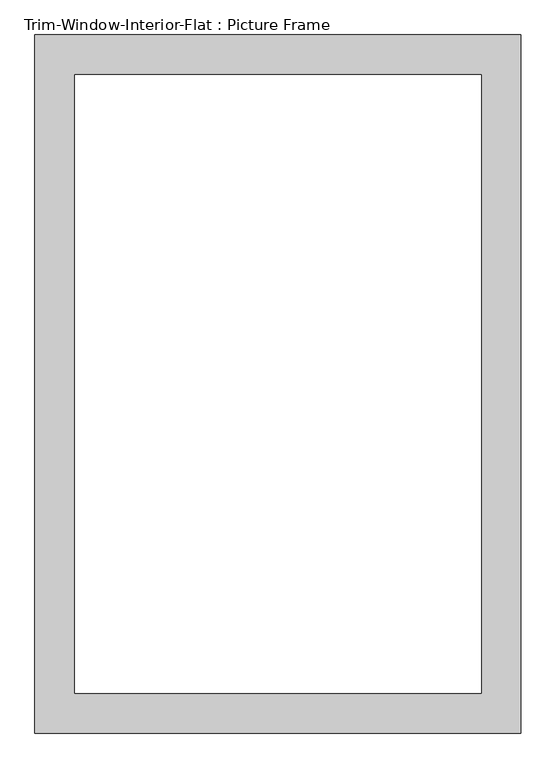
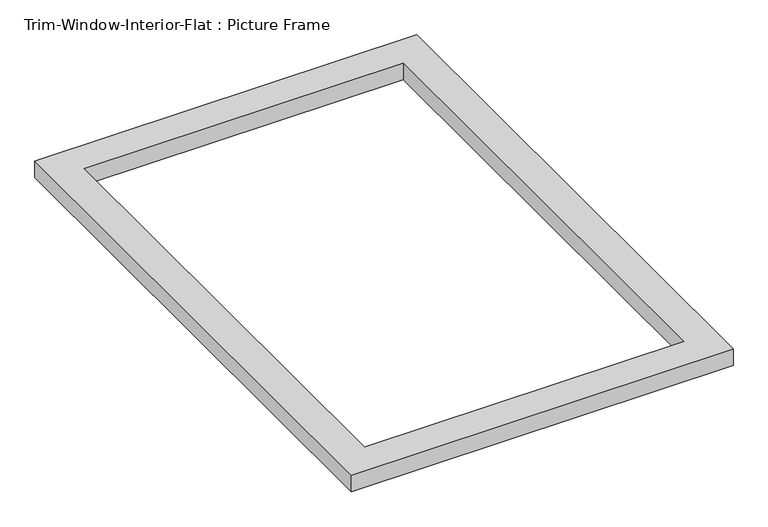
"""IFC4 building model written with IfcOpenShell, lengths in millimetres: proxy geometry, Trim-Window-Interior-Flat : Picture Frame."""

from ifc_helpers import new_model, si_unit, origin, origin_with_axes, place, context, project, spatial, polyline, outline, extrude, source, transform, mapped, element, save


def trim_window_interior_flat_picture_frame_dfd23ff3(model_context):
    return source(origin(), model_context, "Body", "SweptSolid", [
        extrude(outline(polyline([(349.25, -44.45), (-349.25, -44.45), (-349.25, 958.85), (349.25, 958.85), (349.25, -44.45)]), holes=[polyline([(292.1, 12.7), (292.1, 901.7), (-292.1, 901.7), (-292.1, 12.7), (292.1, 12.7)])]), origin_with_axes(), (0.0, 0.0, 1.0), 31.75),
    ])


if __name__ == "__main__":
    model = new_model("IFC4")
    model_context = context("Model", 3, world=origin())
    ifc_project = project(units=[si_unit("LENGTHUNIT", "METRE", prefix="MILLI")], contexts=[model_context])
    site = spatial("IfcSite", under=ifc_project)
    building = spatial("IfcBuilding", under=site)
    placement = place(None, origin())
    trim_window_interior_flat_picture_frame_shape = trim_window_interior_flat_picture_frame_dfd23ff3(model_context)
    element("IfcBuildingElementProxy", 1, Name="Trim-Window-Interior-Flat : Picture Frame", ObjectType="Trim-Window-Interior-Flat : Picture Frame", at=placement, inside=building, context=model_context, shape_type="MappedRepresentation", body=[
        mapped(trim_window_interior_flat_picture_frame_shape, transform((0.0, 0.0, 0.0), x_axis=(1.0, 0.0, 0.0), y_axis=(0.0, 1.0, 0.0), z_axis=(0.0, 0.0, 1.0))),
    ])
    save(model, "model.ifc")

# Revit data of these elements
# Type "Trim-Window-Interior-Flat : Picture Frame"
#   Trim Thickness_Picture Frame = 0' - 1 1/4"
#   Trim Width = 0' - 2 1/4"
#   Trim Thickness_with Sill = 0' - 0 3/4"
#   Sill Thickness = 0' - 1 1/4"
#   Opening Width [instance default] = 2' - 0"
#   Opening Height [instance default] = 3' - 0"
#   Default Elevation = 4' - 0"
#   Sill = no
#   Picture Frame = yes
#   Trim Material [instance default] = none
# Element 1 (IfcBuildingElementProxy, "Trim-Window-Interior-Flat : Picture Frame")
#   Trim Material = Wood - Stained
#   Materials on its faces: "Wood - Stained"
# Materials
#   "Wood - Stained": class "Wood", colour RGB 224 178 126, transparency 0, Cost = 0
